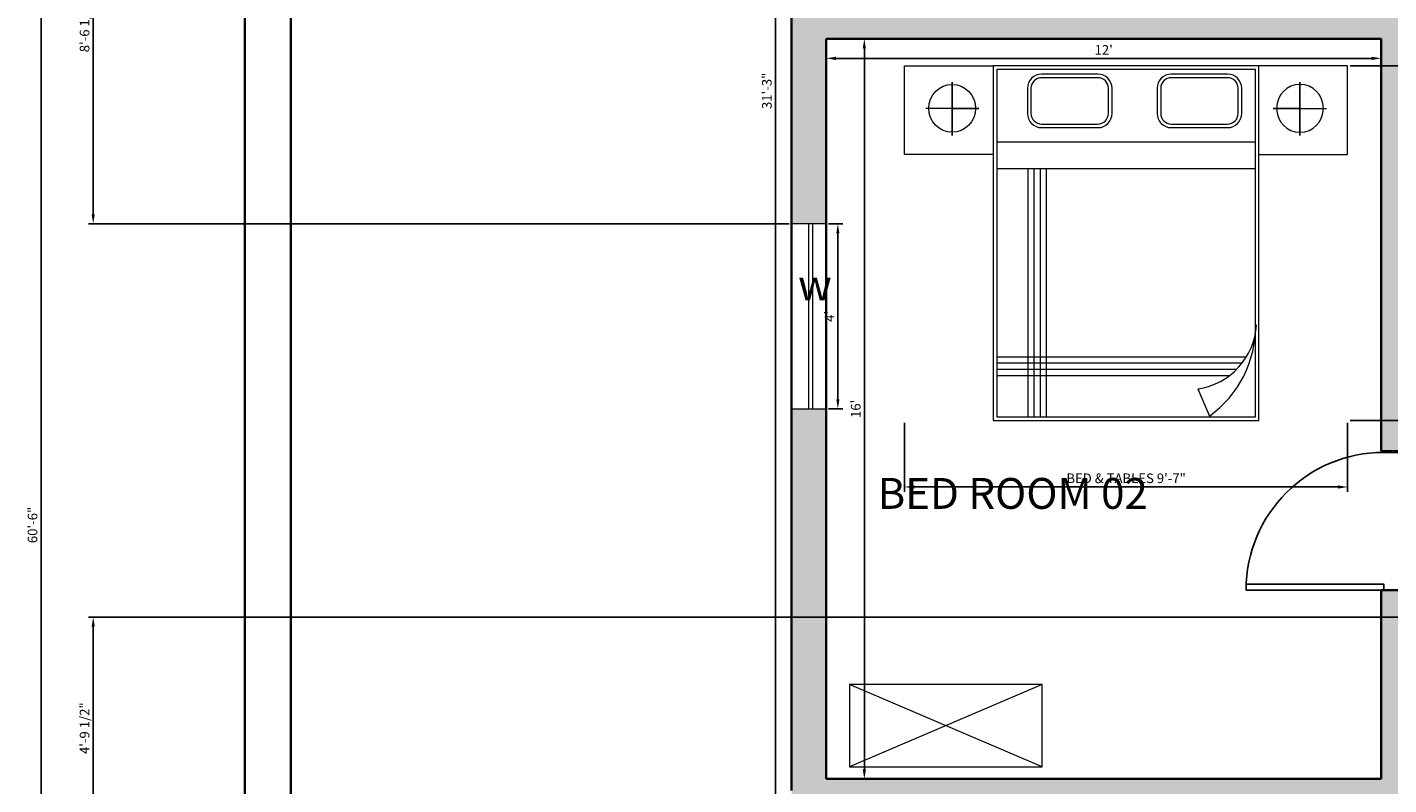
# Model space of a CAD drawing. Units: inches. Extents: x 2901 to 5923, y 918 to 2827.
# Tile 2 of 16: x 4232 to 4585, y 1254 to 1450. Entities that reach past the tile are written whole.
import ezdxf

# ---------------------------------------------------------------- set-up
doc = ezdxf.new("R2010")
doc.units = ezdxf.units.IN
for name, color, linetype, lineweight in [('A-ANNO-DIMS', 2, 'Continuous', 18), ('A-ANNO-TEXT', 7, 'Continuous', 18), ('A-AREA-IDEN', 7, 'Continuous', 25), ('A-GLAZ', 4, 'Continuous', 18), ('A-WALL-PATT', 7, 'Continuous', 13), ('C-PROP', 7, 'Continuous', 35), ('doors', 240, 'Continuous', 25), ('furniture', 160, 'Continuous', 18), ('walls', 7, 'Continuous', 35)]:
    doc.layers.add(name, color=color, linetype=linetype, lineweight=lineweight)
doc.styles.get("Standard").update_dxf_attribs({"font": 'arial.ttf'})
doc.dimstyles.new('Copy of ISO-25', dxfattribs={"dimtxt": 2.5, "dimasz": 2.5, "dimexe": 1.25, "dimexo": 0.625, "dimtad": 1, "dimdec": 1, "dimlunit": 4, "dimtxsty": 'Standard', "dimcen": 2.5, "dimadec": 0, "dimazin": 0, "dimtfac": 1, "dimtdec": 1, "dimtmove": 0, "dimatfit": 3, "dimfxl": 1, "dimarcsym": 0})

# ---------------------------------------------------------------- blocks, each defined once
blk = doc.blocks.new('*U6')
for p, q in [((0, 0), (0, -6)), ((40, 0), (40, -6))]:
    blk.add_line(p, q)
blk.add_lwpolyline([(0, 0), (0, 40), (1.75, 40), (1.75, 0)], close=True)
blk.add_arc((0, 0), 40, 0, 90)
blk = doc.blocks.new('A$C057D194F')
for p, q in [((0, 1.5, -0.1688), (0, 2, -0.1688)), ((0, 2, -0.1688), (0.5, 2, -0.1688)), ((0.5, 2, -0.1688), (0.5, 0, -0.1688)), ((2, 2, -0.1688), (0.5, 2, -0.1688)), ((2, 0, -0.1688), (2, 2, -0.1688)), ((2.5, 2, -0.1688), (2, 2, -0.1688)), ((2.5, 1.5, -0.1688), (2.5, 2, -0.1688)), ((1.98, 1.98, -0.1688), (0.52, 1.98, -0.1688)), ((0.52, 1.98, -0.1688), (0.52, 0.02, -0.1688)), ((1.0907, 1.9539, -0.1688), (0.7735, 1.9539, -0.1688)), ((1.0907, 1.9339, -0.1688), (0.7735, 1.9339, -0.1688)), ((1.8224, 1.9539, -0.1688), (1.5052, 1.9539, -0.1688)), ((1.8224, 1.9339, -0.1688), (1.5052, 1.9339, -0.1688)), ((1.98, 0.02, -0.1688), (1.98, 1.98, -0.1688)), ((0.2687, 1.9081, -0.1688), (0.2687, 1.761, -0.1688)), ((0.2687, 1.6081, -0.1688), (0.2687, 1.9081, -0.1688)), ((0.6935, 1.8739, -0.1688), (0.6935, 1.7322, -0.1688)), ((0.7135, 1.8739, -0.1688), (0.7135, 1.7322, -0.1688)), ((1.1507, 1.7322, -0.1688), (1.1507, 1.8739, -0.1688)), ((1.1707, 1.7322, -0.1688), (1.1707, 1.8739, -0.1688)), ((1.4252, 1.8739, -0.1688), (1.4252, 1.7322, -0.1688)), ((1.4452, 1.8739, -0.1688), (1.4452, 1.7322, -0.1688)), ((1.8824, 1.7322, -0.1688), (1.8824, 1.8739, -0.1688)), ((1.9024, 1.7322, -0.1688), (1.9024, 1.8739, -0.1688)), ((2.2313, 1.9081, -0.1688), (2.2313, 1.761, -0.1688)), ((2.2313, 1.6081, -0.1688), (2.2313, 1.9081, -0.1688)), ((0.4194, 1.761, -0.1688), (0.1194, 1.761, -0.1688)), ((0.2687, 1.761, -0.1688), (0.4194, 1.761, -0.1688)), ((0.2687, 1.761, -0.1688), (0.2687, 1.6081, -0.1688)), ((2.0806, 1.761, -0.1688), (2.3806, 1.761, -0.1688)), ((2.2313, 1.761, -0.1688), (2.0806, 1.761, -0.1688)), ((2.2313, 1.761, -0.1688), (2.2313, 1.6081, -0.1688)), ((0.7735, 1.6722, -0.1688), (1.0907, 1.6722, -0.1688)), ((0.7735, 1.6522, -0.1688), (1.0907, 1.6522, -0.1688)), ((1.5052, 1.6722, -0.1688), (1.8224, 1.6722, -0.1688)), ((1.5052, 1.6522, -0.1688), (1.8224, 1.6522, -0.1688)), ((1.98, 1.5693, -0.1688), (0.52, 1.5693, -0.1688)), ((0.5, 1.5, -0.1688), (0, 1.5, -0.1688)), ((2, 1.5, -0.1688), (2.5, 1.5, -0.1688)), ((1.98, 1.4193, -0.1688), (0.52, 1.4193, -0.1688)), ((0.6969, 0.02, -0.1688), (0.6969, 1.4193, -0.1688)), ((0.7319, 0.02, -0.1688), (0.7319, 1.4193, -0.1688)), ((0.7669, 0.02, -0.1688), (0.7669, 1.4193, -0.1688)), ((0.8019, 0.02, -0.1688), (0.8019, 1.4193, -0.1688)), ((0.52, 0.3595, -0.1688), (1.9292, 0.3595, -0.1688)), ((0.52, 0.3245, -0.1688), (1.905, 0.3245, -0.1688)), ((0.52, 0.2895, -0.1688), (1.8742, 0.2895, -0.1688)), ((0.52, 0.2545, -0.1688), (1.8344, 0.2545, -0.1688)), ((1.6548, 0.1789, -0.1688), (1.7198, 0.0251, -0.1688)), ((0.52, 0.02, -0.1688), (1.98, 0.02, -0.1688)), ((0.5, 0, -0.1688), (2, 0, -0.1688))]:
    blk.add_line(p, q)
for centre, radius, start, end in [((0.7735, 1.8739, -0.1688), 0.08, 90, 180), ((0.7735, 1.8739, -0.1688), 0.06, 90, 180), ((1.0907, 1.8739, -0.1688), 0.08, 0, 90), ((1.0907, 1.8739, -0.1688), 0.06, 0, 90), ((1.5052, 1.8739, -0.1688), 0.08, 90, 180), ((1.5052, 1.8739, -0.1688), 0.06, 90, 180), ((1.8224, 1.8739, -0.1688), 0.08, 0, 90), ((1.8224, 1.8739, -0.1688), 0.06, 0, 90), ((0.7735, 1.7322, -0.1688), 0.08, 180, 270), ((0.7735, 1.7322, -0.1688), 0.06, 180, 270), ((1.0907, 1.7322, -0.1688), 0.08, 270, 0), ((1.0907, 1.7322, -0.1688), 0.06, 270, 0), ((1.5052, 1.7322, -0.1688), 0.08, 180, 270), ((1.5052, 1.7322, -0.1688), 0.06, 180, 270), ((1.8224, 1.7322, -0.1688), 0.08, 270, 0), ((1.8224, 1.7322, -0.1688), 0.06, 270, 0), ((1.5992, 0.5623, -0.1688), 0.3874, 278.2518, 356.6808), ((1.363, 0.5286, -0.1688), 0.6171, 305.32946, 1.04595)]:
    blk.add_arc(centre, radius, start, end)
blk.add_ellipse((0.2687, 1.761, -0.1688), major_axis=(0, -0.1351), ratio=0.975448)
at = {"extrusion": (0, 0, -1)}
blk.add_ellipse((2.2313, 1.761, -0.1688), major_axis=(0, 0.1351), ratio=0.975448, dxfattribs=at)
for p in [(0.2687, 1.761, -0.1688), (2.2313, 1.761, -0.1688)]:
    blk.add_point(p)
blk = doc.blocks.new('*U19')
for p, q in [((0, 0), (38, 89)), ((38, 0), (0, 89))]:
    blk.add_line(p, q)
blk.add_lwpolyline([(0, 0), (38, 0), (38, 89), (0, 89)], close=True)
blk = doc.blocks.new('*D24')
at = {"layer": 'A-ANNO-DIMS', "color": 0, "lineweight": -2, "transparency": 16777216}
for p, q in [((4287.55, 1684.29), (4234.11, 1684.29)), ((4235.36, 1681.79), (4235.36, 960.79)), ((4287.55, 958.29), (4234.11, 958.29))]:
    blk.add_line(p, q, dxfattribs=at)
at = {"layer": 'A-ANNO-DIMS', "color": 0, "transparency": 16777216}
for points in [[(4234.95, 1681.79), (4235.78, 1681.79), (4235.36, 1684.29)], [(4234.95, 960.79), (4235.78, 960.79), (4235.36, 958.29)]]:
    blk.add_solid(points, dxfattribs=at)
at = {"layer": 'Defpoints', "color": 0, "transparency": 16777216}
for p in [(4288.18, 1684.29), (4235.36, 958.29), (4288.18, 958.29)]:
    blk.add_point(p, dxfattribs=at)
at = {"layer": 'A-ANNO-DIMS', "color": 0, "transparency": 16777216, "insert": (4233.46, 1321.29), "char_height": 2.5, "attachment_point": 5, "rotation": 90}
blk.add_mtext('60\'-6"', dxfattribs=at)
blk = doc.blocks.new('*D27')
at = {"layer": 'A-ANNO-DIMS', "color": 0, "lineweight": -2, "transparency": 16777216}
for p, q in [((4429.44, 1621.4), (4424.64, 1621.4)), ((4425.89, 1618.9), (4425.89, 1248.9)), ((4429.44, 1246.4), (4424.64, 1246.4))]:
    blk.add_line(p, q, dxfattribs=at)
at = {"layer": 'A-ANNO-DIMS', "color": 0, "transparency": 16777216}
for points in [[(4425.47, 1618.9), (4426.31, 1618.9), (4425.89, 1621.4)], [(4425.47, 1248.9), (4426.31, 1248.9), (4425.89, 1246.4)]]:
    blk.add_solid(points, dxfattribs=at)
at = {"layer": 'Defpoints', "color": 0, "transparency": 16777216}
for p in [(4430.07, 1621.4), (4425.89, 1246.4), (4430.07, 1246.4)]:
    blk.add_point(p, dxfattribs=at)
at = {"layer": 'A-ANNO-DIMS', "color": 0, "transparency": 16777216, "insert": (4423.99, 1433.9), "char_height": 2.5, "attachment_point": 5, "rotation": 90}
blk.add_mtext('31\'-3"', dxfattribs=at)
blk = doc.blocks.new('*D41')
at = {"layer": 'A-ANNO-DIMS', "color": 0, "lineweight": -2, "transparency": 16777216}
for p, q in [((4439.07, 1446.77), (4439.07, 1441.08)), ((4583.07, 1446.77), (4583.07, 1441.08)), ((4441.57, 1442.33), (4580.57, 1442.33))]:
    blk.add_line(p, q, dxfattribs=at)
at = {"layer": 'A-ANNO-DIMS', "color": 0, "transparency": 16777216}
for points in [[(4441.57, 1442.75), (4441.57, 1441.91), (4439.07, 1442.33)], [(4580.57, 1442.75), (4580.57, 1441.91), (4583.07, 1442.33)]]:
    blk.add_solid(points, dxfattribs=at)
at = {"layer": 'Defpoints', "color": 0, "transparency": 16777216}
for p in [(4439.07, 1447.4), (4583.07, 1447.4), (4583.07, 1442.33)]:
    blk.add_point(p, dxfattribs=at)
at = {"layer": 'A-ANNO-DIMS', "color": 0, "transparency": 16777216, "insert": (4511.07, 1444.21), "char_height": 2.5, "attachment_point": 5}
blk.add_mtext("12'", dxfattribs=at)
blk = doc.blocks.new('*D42')
at = {"layer": 'A-ANNO-DIMS', "color": 0, "lineweight": -2, "transparency": 16777216}
for p, q in [((4439.69, 1447.4), (4450.21, 1447.4)), ((4448.96, 1257.9), (4448.96, 1444.9)), ((4439.69, 1255.4), (4450.21, 1255.4))]:
    blk.add_line(p, q, dxfattribs=at)
at = {"layer": 'A-ANNO-DIMS', "color": 0, "transparency": 16777216}
for points in [[(4448.54, 1444.9), (4449.37, 1444.9), (4448.96, 1447.4)], [(4448.54, 1257.9), (4449.37, 1257.9), (4448.96, 1255.4)]]:
    blk.add_solid(points, dxfattribs=at)
at = {"layer": 'Defpoints', "color": 0, "transparency": 16777216}
for p in [(4439.07, 1447.4), (4448.96, 1447.4), (4439.07, 1255.4)]:
    blk.add_point(p, dxfattribs=at)
at = {"layer": 'A-ANNO-DIMS', "color": 0, "transparency": 16777216, "insert": (4447.06, 1351.4), "char_height": 2.5, "attachment_point": 5, "rotation": 90}
blk.add_mtext("16'", dxfattribs=at)
blk = doc.blocks.new('*D68')
at = {"layer": 'A-ANNO-DIMS', "color": 0, "lineweight": -2, "transparency": 16777216}
for p, q in [((4439.69, 1399.4), (4443.34, 1399.4)), ((4442.09, 1396.9), (4442.09, 1353.9)), ((4439.69, 1351.4), (4443.34, 1351.4))]:
    blk.add_line(p, q, dxfattribs=at)
at = {"layer": 'A-ANNO-DIMS', "color": 0, "transparency": 16777216}
for points in [[(4441.68, 1396.9), (4442.51, 1396.9), (4442.09, 1399.4)], [(4441.68, 1353.9), (4442.51, 1353.9), (4442.09, 1351.4)]]:
    blk.add_solid(points, dxfattribs=at)
at = {"layer": 'Defpoints', "color": 0, "transparency": 16777216}
for p in [(4439.07, 1399.4), (4439.07, 1351.4), (4442.09, 1351.4)]:
    blk.add_point(p, dxfattribs=at)
at = {"layer": 'A-ANNO-DIMS', "color": 0, "transparency": 16777216, "insert": (4440.22, 1375.4), "char_height": 2.5, "attachment_point": 5, "rotation": 90}
blk.add_mtext("4'", dxfattribs=at)
blk = doc.blocks.new('WIN-48')
for p, q in [((0, 9), (0, 0)), ((48, 0), (48, 9)), ((48, 5.5), (0, 5.5)), ((48, 4.5), (0, 4.5))]:
    blk.add_line(p, q)
blk = doc.blocks.new('*D79')
at = {"layer": 'A-ANNO-DIMS', "color": 0, "lineweight": -2, "transparency": 16777216}
for p, q in [((4459.39, 1347.76), (4459.39, 1329.89)), ((4574.36, 1347.76), (4574.36, 1329.89)), ((4461.89, 1331.14), (4571.86, 1331.14))]:
    blk.add_line(p, q, dxfattribs=at)
at = {"layer": 'A-ANNO-DIMS', "color": 0, "transparency": 16777216}
for points in [[(4461.89, 1331.56), (4461.89, 1330.72), (4459.39, 1331.14)], [(4571.86, 1331.56), (4571.86, 1330.72), (4574.36, 1331.14)]]:
    blk.add_solid(points, dxfattribs=at)
at = {"layer": 'Defpoints', "color": 0, "transparency": 16777216}
for p in [(4459.39, 1348.38), (4574.36, 1348.38), (4574.36, 1331.14)]:
    blk.add_point(p, dxfattribs=at)
at = {"layer": 'A-ANNO-DIMS', "color": 0, "transparency": 16777216, "insert": (4516.88, 1333.07), "char_height": 2.5, "attachment_point": 5}
blk.add_mtext('BED & TABLES 9\'-7"', dxfattribs=at)
blk = doc.blocks.new('*D80')
at = {"layer": 'A-ANNO-DIMS', "color": 0, "lineweight": -2, "transparency": 16777216}
for p, q in [((4574.98, 1440.35), (4592.85, 1440.35)), ((4591.6, 1350.88), (4591.6, 1437.85)), ((4574.98, 1348.38), (4592.85, 1348.38))]:
    blk.add_line(p, q, dxfattribs=at)
at = {"layer": 'A-ANNO-DIMS', "color": 0, "transparency": 16777216}
for points in [[(4591.18, 1437.85), (4592.02, 1437.85), (4591.6, 1440.35)], [(4591.18, 1350.88), (4592.02, 1350.88), (4591.6, 1348.38)]]:
    blk.add_solid(points, dxfattribs=at)
at = {"layer": 'Defpoints', "color": 0, "transparency": 16777216}
for p in [(4574.36, 1440.35), (4591.6, 1440.35), (4574.36, 1348.38)]:
    blk.add_point(p, dxfattribs=at)
at = {"layer": 'A-ANNO-DIMS', "color": 0, "transparency": 16777216, "insert": (4589.7, 1394.37), "char_height": 2.5, "attachment_point": 5, "rotation": 90}
blk.add_mtext('7\'-8"', dxfattribs=at)
blk = doc.blocks.new('*D95')
at = {"layer": 'A-ANNO-DIMS', "color": 0, "lineweight": -2, "transparency": 16777216}
for p, q in [((4429.44, 1501.84), (4247.63, 1501.84)), ((4248.88, 1499.34), (4248.88, 1401.9)), ((4429.44, 1399.4), (4247.63, 1399.4))]:
    blk.add_line(p, q, dxfattribs=at)
at = {"layer": 'A-ANNO-DIMS', "color": 0, "transparency": 16777216}
for points in [[(4248.46, 1499.34), (4249.3, 1499.34), (4248.88, 1501.84)], [(4248.46, 1401.9), (4249.3, 1401.9), (4248.88, 1399.4)]]:
    blk.add_solid(points, dxfattribs=at)
at = {"layer": 'Defpoints', "color": 0, "transparency": 16777216}
for p in [(4430.07, 1501.84), (4248.88, 1399.4), (4430.07, 1399.4)]:
    blk.add_point(p, dxfattribs=at)
at = {"layer": 'A-ANNO-DIMS', "color": 0, "transparency": 16777216, "insert": (4246.96, 1450.62), "char_height": 2.5, "attachment_point": 5, "rotation": 90}
blk.add_mtext('8\'-6 1/2"', dxfattribs=at)
blk = doc.blocks.new('*D106')
at = {"layer": 'A-ANNO-DIMS', "color": 0, "lineweight": -2, "transparency": 16777216}
for p, q in [((4588.44, 1297.4), (4247.63, 1297.4)), ((4248.88, 1294.9), (4248.88, 1242.24)), ((4651.2, 1239.74), (4247.63, 1239.74))]:
    blk.add_line(p, q, dxfattribs=at)
at = {"layer": 'A-ANNO-DIMS', "color": 0, "transparency": 16777216}
for points in [[(4248.46, 1294.9), (4249.3, 1294.9), (4248.88, 1297.4)], [(4248.46, 1242.24), (4249.3, 1242.24), (4248.88, 1239.74)]]:
    blk.add_solid(points, dxfattribs=at)
at = {"layer": 'Defpoints', "color": 0, "transparency": 16777216}
for p in [(4589.07, 1297.4), (4248.88, 1239.74), (4651.83, 1239.74)]:
    blk.add_point(p, dxfattribs=at)
at = {"layer": 'A-ANNO-DIMS', "color": 0, "transparency": 16777216, "insert": (4246.96, 1268.57), "char_height": 2.5, "attachment_point": 5, "rotation": 90}
blk.add_mtext('4\'-9 1/2"', dxfattribs=at)

msp = doc.modelspace()

# ---------------------------------------------------------------- hatches: boundary and pattern name
at = {"layer": 'A-WALL-PATT'}
h = msp.add_hatch(color=256, dxfattribs=at)
h.dxf.hatch_style = 1
h.paths.add_polyline_path([(4439.07, 1447.4), (4583.07, 1447.4), (4583.07, 1340.4), (4589.07, 1340.4), (4589.07, 1453.4), (4589.07, 1455.39), (4583.07, 1455.39), (4583.07, 1453.4), (4439.07, 1453.4), (4439.07, 1501.84), (4430.07, 1501.84), (4430.07, 1399.4), (4439.07, 1399.4)])
h.paths.add_polyline_path([(4439.07, 1621.4), (4487.07, 1621.4), (4487.07, 1630.4), (4430.07, 1630.4), (4430.07, 1561.84), (4439.07, 1561.84)])
h.paths.add_polyline_path([(4630.61, 1630.4), (4535.07, 1630.4), (4535.07, 1621.4), (4583.07, 1621.4), (4583.07, 1495.4), (4589.07, 1495.4), (4637.07, 1495.4), (4637.07, 1501.4), (4589.07, 1501.4), (4589.07, 1621.4), (4630.61, 1621.4)])
h.paths.add_polyline_path([(4892.07, 1630.4), (4690.61, 1630.4), (4690.61, 1621.4), (4733.07, 1621.4), (4733.07, 1564.4), (4739.07, 1564.4), (4739.07, 1621.4), (4883.07, 1621.4), (4883.07, 1528.4), (4739.07, 1528.4), (4733.07, 1528.4), (4733.07, 1501.4), (4685.07, 1501.4), (4685.07, 1495.4), (4739.07, 1495.4), (4739.07, 1519.4), (4787.07, 1519.4), (4787.07, 1423.4), (4739.07, 1423.4), (4739.07, 1456.67), (4733.07, 1456.67), (4733.07, 1340.4), (4739.07, 1340.4), (4739.07, 1417.4), (4787.07, 1417.4), (4793.07, 1417.4), (4793.07, 1423.4), (4793.07, 1519.4), (4883.07, 1519.4), (4883.07, 1482.87), (4892.07, 1482.87)])
h.paths.add_polyline_path([(4892.07, 1458.87), (4883.07, 1458.87), (4883.07, 1423.4), (4823.07, 1423.4), (4823.07, 1417.4), (4883.07, 1417.4), (4883.07, 1363.31), (4892.07, 1363.31)], flags=17)
h.paths.add_polyline_path([(4892.07, 1303.31), (4883.07, 1303.31), (4883.07, 1255.4), (4739.07, 1255.4), (4739.07, 1304.4), (4733.07, 1304.4), (4733.07, 1303.4), (4733.07, 1297.4), (4733.07, 1255.4), (4733.07, 1248.4), (4811.07, 1248.4), (4811.07, 1212.16), (4820.07, 1212.16), (4820.07, 1248.4), (4892.07, 1248.4)])
h.paths.add_polyline_path([(4820.07, 1182.16), (4811.07, 1182.16), (4811.07, 1152.4), (4685.07, 1152.4), (4685.07, 1147.03), (4685.07, 1143.4), (4733.07, 1143.4), (4811.07, 1143.4), (4814.07, 1143.4), (4820.07, 1143.4)])
h.paths.add_polyline_path([(4637.07, 1152.4), (4589.07, 1152.4), (4589.07, 1153.4), (4583.86, 1153.4), (4583.07, 1153.4), (4583.07, 1152.4), (4511.07, 1152.4), (4511.07, 1182.16), (4502.07, 1182.16), (4502.07, 1143.4), (4568.07, 1143.4), (4583.07, 1143.4), (4583.07, 1023.4), (4739.07, 1023.4), (4739.07, 1143.4), (4733.07, 1143.4), (4733.07, 1029.4), (4589.07, 1029.4), (4589.07, 1143.4), (4637.07, 1143.4), (4637.07, 1146.97)])
h.paths.add_polyline_path([(4511.07, 1246.4), (4583.07, 1246.4), (4583.07, 1188.4), (4589.07, 1188.4), (4589.07, 1246.4), (4589.07, 1248.4), (4589.07, 1255.4), (4589.07, 1297.4), (4697.07, 1297.4), (4697.07, 1303.4), (4589.07, 1303.4), (4589.07, 1304.4), (4583.07, 1304.4), (4583.07, 1255.4), (4439.07, 1255.4), (4439.07, 1261.4), (4439.07, 1351.4), (4430.07, 1351.4), (4430.07, 1252.4), (4430.07, 1246.4), (4439.07, 1246.4), (4487.07, 1246.4), (4502.07, 1246.4), (4502.07, 1212.16), (4511.07, 1212.16)])

# ---------------------------------------------------------------- linework, layer by layer
at = {"layer": 'A-GLAZ'}
msp.add_line((4430.07, 1399.4), (4430.07, 1351.4), dxfattribs=at)
at = {"layer": 'C-PROP'}
msp.add_lwpolyline([(4288.18, 1684.29), (5015.18, 1684.29), (5015.18, 958.29), (4288.18, 958.29)], close=True, dxfattribs=at)
msp.add_lwpolyline([(5003.18, 978.26), (5003.18, 970.29), (4300.18, 970.29), (4300.18, 1672.29), (5003.18, 1672.29), (5003.18, 1132.27)], dxfattribs=at)
at = {"layer": 'walls'}
for p, q in [((4583.07, 1447.4), (4439.07, 1447.4)), ((4439.07, 1447.4), (4439.07, 1399.4)), ((4583.07, 1447.4), (4583.07, 1340.4)), ((4583.07, 1340.4), (4589.07, 1340.4)), ((4589.07, 1304.4), (4583.07, 1304.4)), ((4583.07, 1304.4), (4583.07, 1255.4)), ((4439.07, 1261.4), (4439.07, 1255.4)), ((4439.07, 1255.4), (4583.07, 1255.4)), ((4439.07, 1255.4), (4487.07, 1255.4))]:
    msp.add_line(p, q, dxfattribs=at)
for points in [[(4892.07, 1630.4), (4430.07, 1630.4), (4430.07, 1252.4)], [(4439.07, 1447.4), (4439.07, 1261.4)]]:
    msp.add_lwpolyline(points, dxfattribs=at)

# ---------------------------------------------------------------- block references
at = {"layer": 'A-GLAZ', "rotation": 269.9999999999979}
msp.add_blockref('WIN-48', (4430.07, 1399.4), dxfattribs=at)
at = {"layer": 'doors', "xscale": 0.8930329219077385, "yscale": 0.8930329219077385, "zscale": 0.8930329219077385, "rotation": 90}
msp.add_blockref('*U6', (4583.71, 1304.4), dxfattribs=at)
at = {"layer": 'furniture', "xscale": 45.98482887225478, "yscale": 45.98482887225478, "zscale": 45.98482887225478}
msp.add_blockref('A$C057D194F', (4459.39, 1348.38, 7.76), dxfattribs=at)
at = {"layer": 'furniture', "xscale": 0.5619183198370973, "yscale": 0.5619183198370973, "zscale": 0.5619183198370973, "rotation": 89.99999999999999}
msp.add_blockref('*U19', (4495.14, 1258.58), dxfattribs=at)

# ---------------------------------------------------------------- texts
at = {"layer": 'A-ANNO-TEXT'}
msp.add_text('w', height=8, dxfattribs=at).set_placement((4431.76, 1379.52))
at = {"layer": 'A-AREA-IDEN'}
msp.add_text('BED ROOM 02', height=8, dxfattribs=at).set_placement((4452.4, 1325.47))

# ---------------------------------------------------------------- dimensions: what is measured, and where the dimension line sits
at = {"layer": 'A-ANNO-DIMS'}
for base, p1, p2, override, picture, middle in [((4235.36, 958.29), (4288.18, 1684.29), (4288.18, 958.29), {"dimclrd": 0, "dimclre": 0, "dimclrt": 0}, '*D24', (4233.46, 1321.29)), ((4425.89, 1246.4), (4430.07, 1621.4), (4430.07, 1246.4), {"dimclrd": 0, "dimclre": 0, "dimclrt": 0}, '*D27', (4423.99, 1433.9)), ((4248.88, 1399.4), (4430.07, 1501.84), (4430.07, 1399.4), {"dimdec": 1, "dimlfac": 1, "dimrnd": 0, "dimzin": 1, "dimdsep": 46, "dimlunit": 4, "dimfrac": 2}, '*D95', (4246.96, 1450.62)), ((4448.96, 1447.4), (4439.07, 1255.4), (4439.07, 1447.4), {"dimclrd": 0, "dimclre": 0, "dimclrt": 0}, '*D42', (4447.06, 1351.4)), ((4591.6, 1440.35), (4574.36, 1348.38), (4574.36, 1440.35), {"dimdec": 1, "dimlfac": 1, "dimrnd": 0, "dimzin": 1, "dimdsep": 46, "dimlunit": 4, "dimfrac": 2}, '*D80', (4589.7, 1394.37)), ((4442.09, 1351.4), (4439.07, 1399.4), (4439.07, 1351.4), {"dimclrd": 0, "dimclre": 0, "dimclrt": 0}, '*D68', (4440.22, 1375.4)), ((4248.88, 1239.74), (4589.07, 1297.4), (4651.83, 1239.74), {"dimdec": 1, "dimlfac": 1, "dimrnd": 0, "dimzin": 1, "dimdsep": 46, "dimlunit": 4, "dimfrac": 2}, '*D106', (4246.96, 1268.57))]:
    dim = msp.add_linear_dim(base=base, p1=p1, p2=p2, angle=90, dimstyle='Copy of ISO-25', override=override, dxfattribs=at)
    dim.commit()
    dim.dimension.update_dxf_attribs({"geometry": picture, "text_midpoint": middle})
dim = msp.add_linear_dim(base=(4583.07, 1442.33), p1=(4439.07, 1447.4), p2=(4583.07, 1447.4), dimstyle='Copy of ISO-25', override={"dimclrd": 0, "dimclre": 0, "dimclrt": 0}, dxfattribs=at)
dim.commit()
dim.dimension.update_dxf_attribs({"geometry": '*D41', "text_midpoint": (4511.07, 1444.21)})
dim = msp.add_linear_dim(base=(4574.36, 1331.14), p1=(4459.39, 1348.38), p2=(4574.36, 1348.38), text='BED & TABLES <>', dimstyle='Copy of ISO-25', override={"dimdec": 1, "dimlfac": 1, "dimrnd": 0, "dimzin": 1, "dimdsep": 46, "dimlunit": 4, "dimfrac": 2}, dxfattribs=at)
dim.commit()
dim.dimension.update_dxf_attribs({"geometry": '*D79', "text_midpoint": (4516.88, 1333.07)})

doc.saveas('drawing.dxf')
